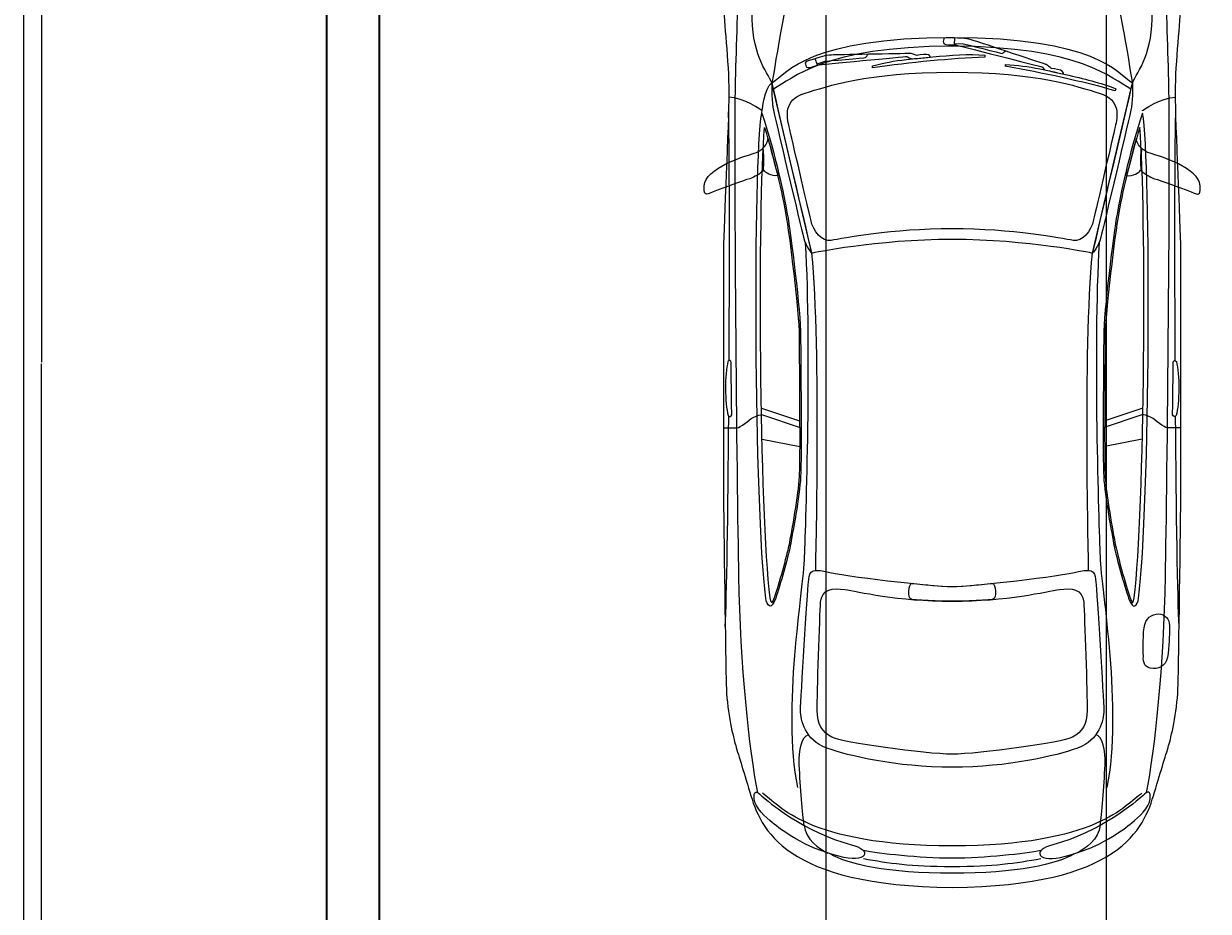
# Model space of a CAD drawing. Units: inches. Extents: x 2460 to 3031, y 933 to 2010.
# Tile 2 of 7: x 2460 to 2663, y 1104 to 1256. Entities that reach past the tile are written whole.
import ezdxf

# ---------------------------------------------------------------- set-up
doc = ezdxf.new("R2010")
doc.units = ezdxf.units.IN
for name, color, linetype, lineweight in [('A-ANNO-DIMS', 2, 'Continuous', 18), ('A-ANNO-TTLB', 7, 'Continuous', 25), ('AUDI', 7, 'Continuous', 25), ('C-PROP', 7, 'Continuous', 35)]:
    doc.layers.add(name, color=color, linetype=linetype, lineweight=lineweight)
doc.styles.get("Standard").update_dxf_attribs({"font": 'arial.ttf'})
doc.dimstyles.get("Standard").update_dxf_attribs({"dimtxt": 0.18, "dimasz": 0.18, "dimexe": 0.18, "dimexo": 0.0625, "dimgap": 0.09, "dimtad": 0, "dimtih": 1, "dimtoh": 1, "dimdec": 4, "dimzin": 0, "dimdsep": 46, "dimtxsty": 'Standard', "dimcen": 0.09, "dimadec": 0, "dimazin": 0, "dimtfac": 1, "dimtdec": 4, "dimtofl": 0, "dimtmove": 0, "dimatfit": 3, "dimfxl": 1, "dimtolj": 1, "dimtzin": 0, "dimarcsym": 0})

# ---------------------------------------------------------------- blocks, each defined once
blk = doc.blocks.new('*D35')
at = {"layer": 'A-ANNO-DIMS', "color": 0, "lineweight": -2, "transparency": 16777216}
for p, q in [((2520.61, 1339.48), (2462.69, 1339.48)), ((2462.87, 1339.3), (2462.87, 1197.91)), ((2462.87, 1056.16), (2462.87, 1197.55)), ((2511.61, 1055.98), (2462.69, 1055.98))]:
    blk.add_line(p, q, dxfattribs=at)
at = {"layer": 'A-ANNO-DIMS', "color": 0, "transparency": 16777216}
for points in [[(2462.84, 1339.3), (2462.9, 1339.3), (2462.87, 1339.48)], [(2462.84, 1056.16), (2462.9, 1056.16), (2462.87, 1055.98)]]:
    blk.add_solid(points, dxfattribs=at)
at = {"layer": 'Defpoints', "color": 0, "transparency": 16777216}
for p in [(2462.87, 1339.48), (2520.67, 1339.48), (2511.67, 1055.98)]:
    blk.add_point(p, dxfattribs=at)
at = {"layer": 'A-ANNO-DIMS', "color": 0, "transparency": 16777216, "insert": (2462.87, 1197.73), "char_height": 0.18, "attachment_point": 5}
blk.add_mtext('\\A1;283.5', dxfattribs=at)
blk = doc.blocks.new('*D37')
at = {"layer": 'A-ANNO-DIMS', "color": 0, "lineweight": -2, "transparency": 16777216}
for p, q in [((2597.17, 1554.98), (2597.17, 933.16)), ((2645.17, 1554.98), (2645.17, 933.16)), ((2597.35, 933.34), (2620.95, 933.34)), ((2644.99, 933.34), (2621.39, 933.34))]:
    blk.add_line(p, q, dxfattribs=at)
at = {"layer": 'A-ANNO-DIMS', "color": 0, "transparency": 16777216}
for points in [[(2597.35, 933.37), (2597.35, 933.31), (2597.17, 933.34)], [(2644.99, 933.37), (2644.99, 933.31), (2645.17, 933.34)]]:
    blk.add_solid(points, dxfattribs=at)
at = {"layer": 'Defpoints', "color": 0, "transparency": 16777216}
for p in [(2597.17, 1555.05), (2645.17, 1555.05), (2645.17, 933.34)]:
    blk.add_point(p, dxfattribs=at)
at = {"layer": 'A-ANNO-DIMS', "color": 0, "transparency": 16777216, "insert": (2621.17, 933.34), "char_height": 0.18, "attachment_point": 5}
blk.add_mtext('\\A1;48', dxfattribs=at)
blk = doc.blocks.new('*D40')
at = {"layer": 'A-ANNO-DIMS', "color": 0, "lineweight": -2, "transparency": 16777216}
for p, q in [((2511.67, 1056.05), (2511.67, 2006.96)), ((2511.85, 2006.78), (2516.02, 2006.78)), ((2520.49, 2006.78), (2516.32, 2006.78)), ((2520.67, 1056.05), (2520.67, 2006.96))]:
    blk.add_line(p, q, dxfattribs=at)
at = {"layer": 'A-ANNO-DIMS', "color": 0, "transparency": 16777216}
for points in [[(2511.85, 2006.81), (2511.85, 2006.75), (2511.67, 2006.78)], [(2520.49, 2006.81), (2520.49, 2006.75), (2520.67, 2006.78)]]:
    blk.add_solid(points, dxfattribs=at)
at = {"layer": 'Defpoints', "color": 0, "transparency": 16777216}
for p in [(2520.67, 2006.78), (2511.67, 1055.98), (2520.67, 1055.98)]:
    blk.add_point(p, dxfattribs=at)
at = {"layer": 'A-ANNO-DIMS', "color": 0, "transparency": 16777216, "insert": (2516.17, 2006.78), "char_height": 0.18, "attachment_point": 5}
blk.add_mtext('\\A1;9', dxfattribs=at)

msp = doc.modelspace()

# ---------------------------------------------------------------- linework, layer by layer
at = {"layer": 'A-ANNO-TTLB'}
msp.add_lwpolyline([(2459.8083, 2009.7942), (3030.6598, 2009.7942), (3030.6598, 936.3732), (2459.8083, 936.3732)], close=True, dxfattribs=at)
at = {"layer": 'AUDI'}
for points, knots in [([(2618.7829, 1107.9984), (2590.0793, 1108.312), (2585.9116, 1117.9641), (2584.1504, 1124.3238), (2584.1504, 1124.3238), (2583.0016, 1128.0786), (2582.0829, 1131.0667), (2581.6233, 1132.5994), (2581.6233, 1132.5994), (2581.1637, 1134.1318), (2580.1686, 1138.8059), (2580.0917, 1142.7138), (2580.0917, 1142.7138), (2580.0148, 1146.6218), (2579.6356, 1169.9218), (2579.6356, 1176.3523), (2579.6356, 1176.3523), (2579.6356, 1182.7825), (2579.6356, 1212.908), (2579.6356, 1217.1935), (2579.6356, 1217.1935), (2579.6356, 1221.4788), (2580.5514, 1238.5719), (2580.5514, 1244.012), (2580.5514, 1244.012), (2580.5514, 1249.4525), (2579.6356, 1256.2783), (2579.6356, 1259.1067), (2579.6356, 1259.1067), (2579.6356, 1261.9354), (2580.1681, 1276.8837), (2580.3981, 1280.1787), (2580.3981, 1280.1787), (2580.6281, 1283.4737), (2581.862, 1285.3424), (2582.9257, 1287.6881), (2582.9257, 1287.6881), (2587.0611, 1296.8058), (2597.6292, 1301.7862), (2598.7781, 1302.5527), (2598.7781, 1302.5527), (2599.9268, 1303.3191), (2601.1463, 1303.7354), (2602.6072, 1303.7354), (2602.6072, 1303.7354), (2604.0679, 1303.7354), (2604.4451, 1303.0127), (2605.0579, 1303.1658), (2605.0579, 1303.1658), (2605.6706, 1303.3191), (2607.1971, 1303.7354), (2608.8874, 1303.7354), (2608.8874, 1303.7354), (2610.5778, 1303.7354), (2618.7829, 1303.7354), (2618.7829, 1303.7354), (2618.7829, 1303.7354), (2618.7829, 1303.7354), (2626.988, 1303.7354), (2628.6784, 1303.7354), (2628.6784, 1303.7354), (2630.3689, 1303.7354), (2631.8952, 1303.3191), (2632.508, 1303.1658), (2632.508, 1303.1658), (2633.1208, 1303.0127), (2633.4979, 1303.7354), (2634.9587, 1303.7354), (2634.9587, 1303.7354), (2636.4196, 1303.7354), (2637.6391, 1303.3191), (2638.7878, 1302.5527), (2638.7878, 1302.5527), (2639.9365, 1301.7863), (2650.5047, 1296.8058), (2654.6402, 1287.6881), (2654.6402, 1287.6881), (2655.7038, 1285.3424), (2656.9377, 1283.4736), (2657.1677, 1280.1787), (2657.1677, 1280.1787), (2657.3978, 1276.8839), (2657.9302, 1261.9353), (2657.9302, 1259.1067), (2657.9302, 1259.1067), (2657.9302, 1256.2784), (2657.0145, 1249.4525), (2657.0145, 1244.012), (2657.0145, 1244.012), (2657.0145, 1238.5719), (2657.9302, 1221.4787), (2657.9302, 1217.1935), (2657.9302, 1217.1935), (2657.9302, 1212.908), (2657.9302, 1182.7824), (2657.9302, 1176.3523), (2657.9302, 1176.3523), (2657.9302, 1169.9218), (2657.5509, 1146.6216), (2657.4742, 1142.7138), (2657.4742, 1142.7138), (2657.3974, 1138.8059), (2656.4022, 1134.1318), (2655.9426, 1132.5994), (2655.9426, 1132.5994), (2655.4829, 1131.0667), (2654.5642, 1128.0785), (2653.4155, 1124.3238), (2653.4155, 1124.3238), (2651.6543, 1117.9641), (2647.4866, 1108.312), (2618.7829, 1107.9984)], [0, 0, 0, 0, 0.03571429, 0.03571429, 0.03571429, 0.0357143, 0.07142857, 0.07142857, 0.07142857, 0.07142858, 0.10714286, 0.10714286, 0.10714286, 0.10714287, 0.14285714, 0.14285714, 0.14285714, 0.14285715, 0.17857143, 0.17857143, 0.17857143, 0.17857144, 0.21428571, 0.21428571, 0.21428571, 0.21428572, 0.25, 0.25, 0.25, 0.25000001, 0.28571429, 0.28571429, 0.28571429, 0.2857143, 0.32142857, 0.32142857, 0.32142857, 0.32142858, 0.35714286, 0.35714286, 0.35714286, 0.35714287, 0.39285714, 0.39285714, 0.39285714, 0.39285715, 0.42857143, 0.42857143, 0.42857143, 0.42857144, 0.46428571, 0.46428571, 0.46428571, 0.46428572, 0.5, 0.5, 0.5, 0.50000001, 0.53571429, 0.53571429, 0.53571429, 0.5357143, 0.57142857, 0.57142857, 0.57142857, 0.57142858, 0.60714286, 0.60714286, 0.60714286, 0.60714287, 0.64285714, 0.64285714, 0.64285714, 0.64285715, 0.67857143, 0.67857143, 0.67857143, 0.67857144, 0.71428571, 0.71428571, 0.71428571, 0.71428572, 0.75, 0.75, 0.75, 0.75000001, 0.78571429, 0.78571429, 0.78571429, 0.7857143, 0.82142857, 0.82142857, 0.82142857, 0.82142858, 0.85714286, 0.85714286, 0.85714286, 0.85714287, 0.89285714, 0.89285714, 0.89285714, 0.89285715, 0.92857143, 0.92857143, 0.92857143, 0.92857144, 0.96428571, 0.96428571, 0.96428571, 0.96428572, 1, 1, 1, 1]), ([(2587.9301, 1245.7186), (2587.0363, 1247.5072), (2584.263, 1251.0766), (2584.5585, 1257.8216), (2584.5585, 1257.8216), (2584.8541, 1264.5669), (2586.0517, 1283.1771), (2587.1263, 1289.0978)], [0, 0, 0, 0, 0.5, 0.5, 0.5, 0.50000001, 1, 1, 1, 1]), ([(2649.6356, 1245.7186), (2650.5296, 1247.5072), (2653.3028, 1251.0766), (2653.0074, 1257.8216), (2653.0074, 1257.8216), (2652.7118, 1264.5669), (2651.5142, 1283.1771), (2650.4396, 1289.0978)], [0, 0, 0, 0, 0.5, 0.5, 0.5, 0.50000001, 1, 1, 1, 1]), ([(2585.4965, 1124.2398), (2584.0544, 1131.455), (2582.5189, 1146.0668), (2582.2566, 1161.2842), (2582.2566, 1161.2842), (2581.9943, 1176.5015), (2581.3391, 1235.0091), (2581.7324, 1247.34), (2581.7324, 1247.34), (2582.1256, 1259.6711), (2582.3457, 1275.227), (2584.5301, 1285.8147)], [0, 0, 0, 0, 0.33333333, 0.33333333, 0.33333333, 0.33333334, 0.66666667, 0.66666667, 0.66666667, 0.66666668, 1, 1, 1, 1]), ([(2652.0694, 1124.2398), (2653.5115, 1131.455), (2655.047, 1146.0668), (2655.3092, 1161.2842), (2655.3092, 1161.2842), (2655.5716, 1176.5015), (2656.2267, 1235.0091), (2655.8335, 1247.34), (2655.8335, 1247.34), (2655.4402, 1259.6711), (2655.2202, 1275.227), (2653.0358, 1285.8147)], [0, 0, 0, 0, 0.33333333, 0.33333333, 0.33333333, 0.33333334, 0.66666667, 0.66666667, 0.66666667, 0.66666668, 1, 1, 1, 1]), ([(2618.7829, 1218.8888), (2631.7756, 1218.8888), (2642.7845, 1216.5384), (2642.7845, 1216.5384), (2642.7845, 1216.5384), (2642.7845, 1216.5384), (2649.6356, 1245.7186), (2649.6356, 1245.7186), (2649.6356, 1245.7186), (2646.895, 1247.4815), (2643.3244, 1253.4548), (2618.7829, 1253.4548), (2618.7829, 1253.4548), (2594.2415, 1253.4548), (2590.6707, 1247.4815), (2587.9303, 1245.7186), (2587.9303, 1245.7186), (2587.9303, 1245.7186), (2594.7813, 1216.5384), (2594.7813, 1216.5384), (2594.7813, 1216.5384), (2594.7813, 1216.5384), (2605.7903, 1218.8886), (2618.7829, 1218.8888)], [0, 0, 0, 0, 0.16666667, 0.16666667, 0.16666667, 0.16666668, 0.33333333, 0.33333333, 0.33333333, 0.33333334, 0.5, 0.5, 0.5, 0.50000001, 0.66666667, 0.66666667, 0.66666667, 0.66666668, 0.83333333, 0.83333333, 0.83333333, 0.83333334, 1, 1, 1, 1]), ([(2618.7829, 1218.8888), (2631.7756, 1218.8888), (2642.7845, 1216.5384), (2642.7845, 1216.5384), (2642.7845, 1216.5384), (2642.7845, 1216.5384), (2649.6356, 1245.7186), (2649.6356, 1245.7186), (2649.6356, 1245.7186), (2646.895, 1247.4815), (2643.3244, 1253.4548), (2618.7829, 1253.4548), (2618.7829, 1253.4548), (2594.2415, 1253.4548), (2590.6707, 1247.4815), (2587.9303, 1245.7186), (2587.9303, 1245.7186), (2587.9303, 1245.7186), (2594.7813, 1216.5384), (2594.7813, 1216.5384), (2594.7813, 1216.5384), (2594.7813, 1216.5384), (2605.7903, 1218.8888), (2618.7829, 1218.8888)], [0, 0, 0, 0, 0.16666667, 0.16666667, 0.16666667, 0.16666668, 0.33333333, 0.33333333, 0.33333333, 0.33333334, 0.5, 0.5, 0.5, 0.50000001, 0.66666667, 0.66666667, 0.66666667, 0.66666668, 0.83333333, 0.83333333, 0.83333333, 0.83333334, 1, 1, 1, 1]), ([(2649.3768, 1244.617), (2646.0401, 1246.3912), (2640.8837, 1251.9486), (2618.7829, 1251.9486), (2618.7829, 1251.9486), (2596.6822, 1251.9486), (2591.5257, 1246.3912), (2588.1891, 1244.6168)], [0, 0, 0, 0, 0.5, 0.5, 0.5, 0.50000001, 1, 1, 1, 1]), ([(2619.672, 1253.3532), (2620.8626, 1253.3532), (2621.7312, 1253.1598), (2622.7614, 1252.8377), (2622.7614, 1252.8377), (2623.5334, 1252.6126), (2634.9246, 1248.8131), (2634.9246, 1248.8131), (2634.9246, 1248.8131), (2634.9246, 1248.8131), (2635.6972, 1248.2013), (2635.6972, 1248.2013), (2635.6972, 1248.2013), (2635.6972, 1248.2013), (2636.7268, 1248.0082), (2637.306, 1247.8799), (2637.306, 1247.8799), (2637.8856, 1247.719), (2637.821, 1247.2034), (2637.821, 1247.2034), (2637.821, 1247.2034), (2637.821, 1247.2034), (2634.6672, 1247.9118), (2634.6672, 1247.9118), (2634.6672, 1247.9118), (2634.6672, 1247.9118), (2634.1526, 1248.4273), (2634.1526, 1248.4273), (2634.1526, 1248.4273), (2634.1526, 1248.4273), (2619.3499, 1252.194), (2619.3499, 1252.194), (2619.3499, 1252.194), (2619.3499, 1252.194), (2618.8671, 1252.1939), (2618.127, 1252.1939), (2618.127, 1252.1939), (2617.3866, 1252.2259), (2617.2584, 1252.4837), (2617.2584, 1252.7731), (2617.2584, 1252.7731), (2617.2584, 1253.0953), (2617.2907, 1253.3855), (2617.7411, 1253.3855), (2617.7411, 1253.3855), (2618.1915, 1253.4175), (2618.9317, 1253.3855), (2619.672, 1253.3532)], [0, 0, 0, 0, 0.08333333, 0.08333333, 0.08333333, 0.08333334, 0.16666667, 0.16666667, 0.16666667, 0.16666668, 0.25, 0.25, 0.25, 0.25000001, 0.33333333, 0.33333333, 0.33333333, 0.33333334, 0.41666667, 0.41666667, 0.41666667, 0.41666668, 0.5, 0.5, 0.5, 0.50000001, 0.58333333, 0.58333333, 0.58333333, 0.58333334, 0.66666667, 0.66666667, 0.66666667, 0.66666668, 0.75, 0.75, 0.75, 0.75000001, 0.83333333, 0.83333333, 0.83333333, 0.83333334, 0.91666667, 0.91666667, 0.91666667, 0.91666668, 1, 1, 1, 1]), ([(2619.1893, 1252.4193), (2619.1893, 1252.4193), (2620.6693, 1252.387), (2620.6693, 1252.387), (2620.6693, 1252.387), (2620.6693, 1252.387), (2627.3624, 1250.7126), (2627.3624, 1250.7126), (2627.3624, 1250.7126), (2627.3624, 1250.7126), (2627.9098, 1251.1312), (2627.9098, 1251.1312)], [0, 0, 0, 0, 0.33333333, 0.33333333, 0.33333333, 0.33333334, 0.66666667, 0.66666667, 0.66666667, 0.66666668, 1, 1, 1, 1]), ([(2595.7944, 1249.972), (2596.8886, 1250.3588), (2597.7895, 1250.455), (2598.8837, 1250.4873), (2598.8837, 1250.4873), (2599.6881, 1250.4875), (2611.7877, 1250.7126), (2611.7877, 1250.7126), (2611.7877, 1250.7126), (2611.7877, 1250.7126), (2612.7208, 1250.3906), (2612.7208, 1250.3906), (2612.7208, 1250.3906), (2612.7208, 1250.3906), (2613.7828, 1250.5197), (2614.362, 1250.552), (2614.362, 1250.552), (2614.9416, 1250.6162), (2615.0376, 1250.1011), (2615.0376, 1250.1011), (2615.0376, 1250.1011), (2615.0376, 1250.1011), (2611.8524, 1249.779), (2611.8524, 1249.779), (2611.8524, 1249.779), (2611.8524, 1249.779), (2610.9834, 1250.1976), (2610.9834, 1250.1976), (2610.9834, 1250.1976), (2610.9834, 1250.1976), (2595.859, 1248.7808), (2595.859, 1248.7808), (2595.859, 1248.7808), (2595.859, 1248.7808), (2595.4086, 1248.6202), (2594.7006, 1248.3949), (2594.7006, 1248.3949), (2594.0245, 1248.1694), (2593.7994, 1248.3626), (2593.7028, 1248.6525), (2593.7028, 1248.6525), (2593.6059, 1248.9738), (2593.5418, 1249.2326), (2593.9604, 1249.3927), (2593.9604, 1249.3927), (2594.3785, 1249.5216), (2595.0864, 1249.7467), (2595.7944, 1249.972)], [0, 0, 0, 0, 0.08333333, 0.08333333, 0.08333333, 0.08333334, 0.16666667, 0.16666667, 0.16666667, 0.16666668, 0.25, 0.25, 0.25, 0.25000001, 0.33333333, 0.33333333, 0.33333333, 0.33333334, 0.41666667, 0.41666667, 0.41666667, 0.41666668, 0.5, 0.5, 0.5, 0.50000001, 0.58333333, 0.58333333, 0.58333333, 0.58333334, 0.66666667, 0.66666667, 0.66666667, 0.66666668, 0.75, 0.75, 0.75, 0.75000001, 0.83333333, 0.83333333, 0.83333333, 0.83333334, 0.91666667, 0.91666667, 0.91666667, 0.91666668, 1, 1, 1, 1]), ([(2595.7944, 1249.972), (2596.8886, 1250.3588), (2597.7895, 1250.455), (2598.8837, 1250.4873), (2598.8837, 1250.4873), (2599.6881, 1250.4873), (2611.7877, 1250.7126), (2611.7877, 1250.7126), (2611.7877, 1250.7126), (2611.7877, 1250.7126), (2612.7208, 1250.3906), (2612.7208, 1250.3906), (2612.7208, 1250.3906), (2612.7208, 1250.3906), (2613.7828, 1250.5197), (2614.362, 1250.552), (2614.362, 1250.552), (2614.9416, 1250.6162), (2615.0376, 1250.1011), (2615.0376, 1250.1011), (2615.0376, 1250.1011), (2615.0376, 1250.1011), (2611.8524, 1249.779), (2611.8524, 1249.779), (2611.8524, 1249.779), (2611.8524, 1249.779), (2610.9834, 1250.1976), (2610.9834, 1250.1976), (2610.9834, 1250.1976), (2610.9834, 1250.1976), (2595.859, 1248.7808), (2595.859, 1248.7808), (2595.859, 1248.7808), (2595.859, 1248.7808), (2595.4086, 1248.6202), (2594.7006, 1248.3949), (2594.7006, 1248.3949), (2594.0245, 1248.1694), (2593.7994, 1248.3626), (2593.7028, 1248.6525), (2593.7028, 1248.6525), (2593.6059, 1248.9738), (2593.5418, 1249.2326), (2593.9604, 1249.3927), (2593.9604, 1249.3927), (2594.3785, 1249.5216), (2595.0864, 1249.7467), (2595.7944, 1249.972)], [0, 0, 0, 0, 0.08333333, 0.08333333, 0.08333333, 0.08333334, 0.16666667, 0.16666667, 0.16666667, 0.16666668, 0.25, 0.25, 0.25, 0.25000001, 0.33333333, 0.33333333, 0.33333333, 0.33333334, 0.41666667, 0.41666667, 0.41666667, 0.41666668, 0.5, 0.5, 0.5, 0.50000001, 0.58333333, 0.58333333, 0.58333333, 0.58333334, 0.66666667, 0.66666667, 0.66666667, 0.66666668, 0.75, 0.75, 0.75, 0.75000001, 0.83333333, 0.83333333, 0.83333333, 0.83333334, 0.91666667, 0.91666667, 0.91666667, 0.91666668, 1, 1, 1, 1]), ([(2595.666, 1248.942), (2595.666, 1248.942), (2597.0492, 1249.3929), (2597.0492, 1249.3929), (2597.0492, 1249.3929), (2597.0492, 1249.3929), (2603.9681, 1250.0043), (2603.9681, 1250.0043), (2603.9681, 1250.0043), (2603.9681, 1250.0043), (2604.3543, 1250.5521), (2604.3543, 1250.5521)], [0, 0, 0, 0, 0.33333333, 0.33333333, 0.33333333, 0.33333334, 0.66666667, 0.66666667, 0.66666667, 0.66666668, 1, 1, 1, 1]), ([(2624.3701, 1250.4552), (2621.6025, 1250.6481), (2618.5774, 1250.4227), (2615.4558, 1250.1334), (2615.4558, 1250.1334), (2613.9439, 1249.972), (2612.4311, 1249.8436), (2610.9511, 1249.6821), (2610.9511, 1249.6821), (2608.8595, 1249.4893), (2607.0897, 1249.0706), (2605.1587, 1248.6202), (2605.1587, 1248.6202), (2605.1587, 1248.6202), (2605.1587, 1248.2654), (2605.1587, 1248.2654), (2605.1587, 1248.2654), (2611.7231, 1249.1999), (2618.5455, 1249.8436), (2624.4024, 1250.1011), (2624.4024, 1250.1011), (2624.4024, 1250.1011), (2624.3701, 1250.4552), (2624.3701, 1250.4552)], [0, 0, 0, 0, 0.16666667, 0.16666667, 0.16666667, 0.16666668, 0.33333333, 0.33333333, 0.33333333, 0.33333334, 0.5, 0.5, 0.5, 0.50000001, 0.66666667, 0.66666667, 0.66666667, 0.66666668, 0.83333333, 0.83333333, 0.83333333, 0.83333334, 1, 1, 1, 1]), ([(2618.7829, 1220.7249), (2629.0961, 1220.7249), (2637.5374, 1219.0336), (2639.4913, 1218.7381), (2639.4913, 1218.7381), (2641.0857, 1218.4968), (2642.5602, 1220.2217), (2643.0071, 1222.29), (2643.0071, 1222.29), (2643.454, 1224.3581), (2646.3033, 1236.4318), (2646.6944, 1238.1647), (2646.6944, 1238.1647), (2647.0855, 1239.8976), (2647.7558, 1242.7484), (2643.9568, 1243.9221), (2643.9568, 1243.9221), (2640.1579, 1245.0962), (2633.4425, 1247.4993), (2618.7829, 1247.4993), (2618.7829, 1247.4993), (2604.1234, 1247.4993), (2597.408, 1245.0961), (2593.6091, 1243.9221), (2593.6091, 1243.9221), (2589.81, 1242.7485), (2590.4804, 1239.8975), (2590.8715, 1238.1647), (2590.8715, 1238.1647), (2591.2625, 1236.432), (2594.1118, 1224.358), (2594.5587, 1222.29), (2594.5587, 1222.29), (2595.0057, 1220.2218), (2596.4801, 1218.4968), (2598.0744, 1218.7381), (2598.0744, 1218.7381), (2600.0285, 1219.0337), (2608.4697, 1220.7249), (2618.7829, 1220.7249)], [0, 0, 0, 0, 0.1, 0.1, 0.1, 0.10000001, 0.2, 0.2, 0.2, 0.20000001, 0.3, 0.3, 0.3, 0.30000001, 0.4, 0.4, 0.4, 0.40000001, 0.5, 0.5, 0.5, 0.50000001, 0.6, 0.6, 0.6, 0.60000001, 0.7, 0.7, 0.7, 0.70000001, 0.8, 0.8, 0.8, 0.80000001, 0.9, 0.9, 0.9, 0.90000001, 1, 1, 1, 1]), ([(2646.7991, 1244.6921), (2644.2248, 1245.6898), (2641.2962, 1246.4304), (2638.2069, 1247.1065), (2638.2069, 1247.1065), (2636.7268, 1247.4286), (2635.2468, 1247.7826), (2633.7986, 1248.0724), (2633.7986, 1248.0724), (2631.7713, 1248.5243), (2629.9368, 1248.6843), (2627.9422, 1248.8454), (2627.9422, 1248.8454), (2627.9422, 1248.8454), (2627.8452, 1248.5243), (2627.8452, 1248.5243), (2627.8452, 1248.5243), (2634.3778, 1247.3965), (2641.0391, 1245.9154), (2646.7026, 1244.338), (2646.7026, 1244.338), (2646.7026, 1244.338), (2646.7991, 1244.6921), (2646.7991, 1244.6921)], [0, 0, 0, 0, 0.16666667, 0.16666667, 0.16666667, 0.16666668, 0.33333333, 0.33333333, 0.33333333, 0.33333334, 0.5, 0.5, 0.5, 0.50000001, 0.66666667, 0.66666667, 0.66666667, 0.66666668, 0.83333333, 0.83333333, 0.83333333, 0.83333334, 1, 1, 1, 1]), ([(2587.9301, 1245.7186), (2587.9301, 1245.7186), (2594.7813, 1216.5384), (2594.7813, 1216.5384), (2594.7813, 1216.5384), (2594.7813, 1216.5384), (2593.7103, 1217.5998), (2593.3188, 1219.2645), (2593.3188, 1219.2645), (2592.9272, 1220.9292), (2588.3828, 1239.9489), (2588.089, 1241.5154), (2588.089, 1241.5154), (2587.7953, 1243.082), (2587.9303, 1245.7186), (2587.9301, 1245.7186)], [0, 0, 0, 0, 0.25, 0.25, 0.25, 0.25000001, 0.5, 0.5, 0.5, 0.50000001, 0.75, 0.75, 0.75, 0.75000001, 1, 1, 1, 1]), ([(2587.9301, 1245.7186), (2587.9301, 1245.7186), (2594.7813, 1216.5384), (2594.7813, 1216.5384), (2594.7813, 1216.5384), (2594.7813, 1216.5384), (2593.7103, 1217.5998), (2593.3188, 1219.2645), (2593.3188, 1219.2645), (2592.9272, 1220.9292), (2588.3828, 1239.9489), (2588.089, 1241.5154), (2588.089, 1241.5154), (2587.7953, 1243.082), (2587.9301, 1245.7186), (2587.9301, 1245.7186)], [0, 0, 0, 0, 0.25, 0.25, 0.25, 0.25000001, 0.5, 0.5, 0.5, 0.50000001, 0.75, 0.75, 0.75, 0.75000001, 1, 1, 1, 1]), ([(2649.6356, 1245.7186), (2649.6356, 1245.7186), (2642.7845, 1216.5384), (2642.7845, 1216.5384), (2642.7845, 1216.5384), (2642.7845, 1216.5384), (2643.8556, 1217.5998), (2644.2471, 1219.2645), (2644.2471, 1219.2645), (2644.6385, 1220.9292), (2649.1831, 1239.9489), (2649.4768, 1241.5154), (2649.4768, 1241.5154), (2649.7706, 1243.082), (2649.6356, 1245.7186), (2649.6356, 1245.7186)], [0, 0, 0, 0, 0.25, 0.25, 0.25, 0.25000001, 0.5, 0.5, 0.5, 0.50000001, 0.75, 0.75, 0.75, 0.75000001, 1, 1, 1, 1]), ([(2586.8744, 1157.4941), (2587.0272, 1156.2939), (2587.7696, 1155.2062), (2588.5648, 1157.4941), (2588.5648, 1157.4941), (2589.3601, 1159.7819), (2590.6525, 1164.4571), (2591.05, 1166.4463), (2591.05, 1166.4463), (2591.4476, 1168.4352), (2592.6409, 1174.9998), (2592.8395, 1178.2823), (2592.8395, 1178.2823), (2593.0382, 1181.5647), (2592.8395, 1198.3743), (2592.8395, 1202.3528), (2592.8395, 1202.3528), (2592.8395, 1206.3316), (2591.1496, 1219.9584), (2590.5529, 1223.2406), (2590.5529, 1223.2406), (2589.9563, 1226.5229), (2588.6639, 1233.0877), (2586.1752, 1240.4823), (2586.1752, 1240.4823), (2584.6877, 1232.2922), (2584.8859, 1173.1101), (2586.8744, 1157.4941)], [0, 0, 0, 0, 0.14285714, 0.14285714, 0.14285714, 0.14285715, 0.28571429, 0.28571429, 0.28571429, 0.2857143, 0.42857143, 0.42857143, 0.42857143, 0.42857144, 0.57142857, 0.57142857, 0.57142857, 0.57142858, 0.71428571, 0.71428571, 0.71428571, 0.71428572, 0.85714286, 0.85714286, 0.85714286, 0.85714287, 1, 1, 1, 1]), ([(2650.6915, 1157.4941), (2650.5387, 1156.2939), (2649.7963, 1155.2062), (2649.001, 1157.4941), (2649.001, 1157.4941), (2648.2058, 1159.7819), (2646.9135, 1164.4571), (2646.5159, 1166.4463), (2646.5159, 1166.4463), (2646.1183, 1168.4352), (2644.9249, 1174.9998), (2644.7263, 1178.2823), (2644.7263, 1178.2823), (2644.5277, 1181.5647), (2644.7263, 1198.3743), (2644.7263, 1202.3528), (2644.7263, 1202.3528), (2644.7263, 1206.3316), (2646.4163, 1219.9584), (2647.013, 1223.2406), (2647.013, 1223.2406), (2647.6096, 1226.5229), (2648.902, 1233.0877), (2651.3907, 1240.4823), (2651.3907, 1240.4823), (2652.8782, 1232.2922), (2652.68, 1173.1101), (2650.6915, 1157.4941)], [0, 0, 0, 0, 0.14285714, 0.14285714, 0.14285714, 0.14285715, 0.28571429, 0.28571429, 0.28571429, 0.2857143, 0.42857143, 0.42857143, 0.42857143, 0.42857144, 0.57142857, 0.57142857, 0.57142857, 0.57142858, 0.71428571, 0.71428571, 0.71428571, 0.71428572, 0.85714286, 0.85714286, 0.85714286, 0.85714287, 1, 1, 1, 1]), ([(2587.6304, 1157.5581), (2587.6304, 1157.5581), (2587.6304, 1157.5581), (2587.6304, 1157.5581), (2587.6304, 1157.5581), (2587.6862, 1157.1186), (2587.8058, 1156.8635), (2587.8926, 1156.7406), (2587.8926, 1156.7406), (2587.9835, 1156.8489), (2588.1402, 1157.0879), (2588.3392, 1157.6607), (2588.3392, 1157.6607), (2589.1143, 1159.8904), (2590.4054, 1164.5405), (2590.806, 1166.5455), (2590.806, 1166.5455), (2591.2862, 1168.9474), (2592.4013, 1175.2447), (2592.5868, 1178.3128), (2592.5868, 1178.3128), (2592.7321, 1180.7132), (2592.6623, 1190.5221), (2592.6164, 1197.013), (2592.6164, 1197.013), (2592.6164, 1197.013), (2592.5859, 1202.3529), (2592.5859, 1202.3529), (2592.5859, 1202.3529), (2592.5859, 1206.3203), (2590.8776, 1220.0125), (2590.3076, 1223.1499), (2590.3076, 1223.1499), (2589.3539, 1228.3963), (2588.117, 1233.392), (2586.654, 1238.0769), (2586.654, 1238.0769), (2585.4851, 1224.5051), (2585.7875, 1172.0275), (2587.6304, 1157.5581)], [0, 0, 0, 0, 0.1, 0.1, 0.1, 0.10000001, 0.2, 0.2, 0.2, 0.20000001, 0.3, 0.3, 0.3, 0.30000001, 0.4, 0.4, 0.4, 0.40000001, 0.5, 0.5, 0.5, 0.50000001, 0.6, 0.6, 0.6, 0.60000001, 0.7, 0.7, 0.7, 0.70000001, 0.8, 0.8, 0.8, 0.80000001, 0.9, 0.9, 0.9, 0.90000001, 1, 1, 1, 1]), ([(2649.9355, 1157.5581), (2649.9355, 1157.5581), (2649.9355, 1157.5581), (2649.9355, 1157.5581), (2649.9355, 1157.5581), (2649.8796, 1157.1186), (2649.76, 1156.8635), (2649.6733, 1156.7406), (2649.6733, 1156.7406), (2649.5824, 1156.8489), (2649.4257, 1157.0879), (2649.2267, 1157.6607), (2649.2267, 1157.6607), (2648.4516, 1159.8904), (2647.1605, 1164.5405), (2646.7599, 1166.5455), (2646.7599, 1166.5455), (2646.2797, 1168.9474), (2645.1646, 1175.2447), (2644.9791, 1178.3128), (2644.9791, 1178.3128), (2644.8337, 1180.7132), (2644.9036, 1190.5221), (2644.9493, 1197.013), (2644.9493, 1197.013), (2644.9493, 1197.013), (2644.98, 1202.3529), (2644.98, 1202.3529), (2644.98, 1202.3529), (2644.98, 1206.3203), (2646.6883, 1220.0125), (2647.2583, 1223.1499), (2647.2583, 1223.1499), (2648.2119, 1228.3963), (2649.4489, 1233.392), (2650.9119, 1238.0769), (2650.9119, 1238.0769), (2652.0808, 1224.5051), (2651.7782, 1172.0275), (2649.9355, 1157.5581)], [0, 0, 0, 0, 0.1, 0.1, 0.1, 0.10000001, 0.2, 0.2, 0.2, 0.20000001, 0.3, 0.3, 0.3, 0.30000001, 0.4, 0.4, 0.4, 0.40000001, 0.5, 0.5, 0.5, 0.50000001, 0.6, 0.6, 0.6, 0.60000001, 0.7, 0.7, 0.7, 0.70000001, 0.8, 0.8, 0.8, 0.80000001, 0.9, 0.9, 0.9, 0.90000001, 1, 1, 1, 1]), ([(2586.341, 1234.4618), (2586.499, 1233.6439), (2586.5135, 1231.8626), (2586.4178, 1230.6365), (2586.4178, 1230.6365), (2586.4532, 1230.6755), (2586.4924, 1230.7151), (2586.5165, 1230.75), (2586.5165, 1230.75), (2586.7364, 1230.283), (2587.8687, 1229.6668), (2588.9096, 1229.8374), (2588.9096, 1229.8374), (2588.773, 1230.4084), (2587.2523, 1236.0998), (2587.2523, 1236.0998), (2587.2523, 1236.0998), (2587.1904, 1235.6289), (2586.894, 1234.9895), (2586.341, 1234.4618)], [0, 0, 0, 0, 0.2, 0.2, 0.2, 0.20000001, 0.4, 0.4, 0.4, 0.40000001, 0.6, 0.6, 0.6, 0.60000001, 0.8, 0.8, 0.8, 0.80000001, 1, 1, 1, 1]), ([(2651.2248, 1234.4618), (2651.0669, 1233.6439), (2651.0524, 1231.8626), (2651.1481, 1230.6365), (2651.1481, 1230.6365), (2651.1127, 1230.6755), (2651.0735, 1230.7151), (2651.0494, 1230.75), (2651.0494, 1230.75), (2650.8294, 1230.283), (2649.6972, 1229.6668), (2648.6563, 1229.8374), (2648.6563, 1229.8374), (2648.7929, 1230.4084), (2650.3136, 1236.0998), (2650.3136, 1236.0998), (2650.3136, 1236.0998), (2650.3755, 1235.6289), (2650.6718, 1234.9895), (2651.2248, 1234.4618)], [0, 0, 0, 0, 0.2, 0.2, 0.2, 0.20000001, 0.4, 0.4, 0.4, 0.40000001, 0.6, 0.6, 0.6, 0.60000001, 0.8, 0.8, 0.8, 0.80000001, 1, 1, 1, 1]), ([(2586.341, 1234.4618), (2585.97, 1234.1074), (2585.4864, 1233.8022), (2584.8684, 1233.6364), (2584.8684, 1233.6364), (2583.3298, 1233.2235), (2576.4075, 1231.0529), (2576.3251, 1228.0841), (2576.3251, 1228.0841), (2576.3251, 1226.8198), (2576.3522, 1226.3801), (2577.3411, 1226.8196), (2577.3411, 1226.8196), (2578.3302, 1227.2596), (2583.3029, 1229.0456), (2584.1269, 1229.2932), (2584.1269, 1229.2932), (2584.8855, 1229.5215), (2586.0071, 1230.1882), (2586.4178, 1230.6365), (2586.4178, 1230.6365), (2586.5135, 1231.8626), (2586.499, 1233.6439), (2586.341, 1234.4618)], [0, 0, 0, 0, 0.16666667, 0.16666667, 0.16666667, 0.16666668, 0.33333333, 0.33333333, 0.33333333, 0.33333334, 0.5, 0.5, 0.5, 0.50000001, 0.66666667, 0.66666667, 0.66666667, 0.66666668, 0.83333333, 0.83333333, 0.83333333, 0.83333334, 1, 1, 1, 1]), ([(2651.2248, 1234.4618), (2651.5958, 1234.1074), (2652.0794, 1233.8022), (2652.6975, 1233.6364), (2652.6975, 1233.6364), (2654.2359, 1233.2235), (2661.1583, 1231.0529), (2661.2408, 1228.0841), (2661.2408, 1228.0841), (2661.2408, 1226.8198), (2661.2137, 1226.3801), (2660.2247, 1226.8196), (2660.2247, 1226.8196), (2659.2357, 1227.2596), (2654.263, 1229.0456), (2653.439, 1229.2932), (2653.439, 1229.2932), (2652.6804, 1229.5215), (2651.5587, 1230.1882), (2651.1481, 1230.6365), (2651.1481, 1230.6365), (2651.0524, 1231.8626), (2651.0669, 1233.6439), (2651.2248, 1234.4618)], [0, 0, 0, 0, 0.16666667, 0.16666667, 0.16666667, 0.16666668, 0.33333333, 0.33333333, 0.33333333, 0.33333334, 0.5, 0.5, 0.5, 0.50000001, 0.66666667, 0.66666667, 0.66666667, 0.66666668, 0.83333333, 0.83333333, 0.83333333, 0.83333334, 1, 1, 1, 1]), ([(2593.6309, 1218.3227), (2594.6596, 1199.7579), (2593.6915, 1170.563), (2593.4681, 1164.638), (2593.4681, 1164.638), (2593.2446, 1158.713), (2589.618, 1138.5888), (2592.2756, 1125.1233)], [0, 0, 0, 0, 0.5, 0.5, 0.5, 0.50000001, 1, 1, 1, 1]), ([(2643.935, 1218.3227), (2642.9063, 1199.7579), (2643.8743, 1170.563), (2644.0978, 1164.638), (2644.0978, 1164.638), (2644.3213, 1158.713), (2647.9479, 1138.5888), (2645.2902, 1125.1233)], [0, 0, 0, 0, 0.5, 0.5, 0.5, 0.50000001, 1, 1, 1, 1]), ([(2581.0384, 1188.9052), (2581.0384, 1188.5544), (2580.5587, 1188.4227), (2580.4523, 1188.7737), (2580.4523, 1188.7737), (2580.1319, 1189.7827), (2579.973, 1191.5807), (2579.973, 1193.3791), (2579.973, 1193.3791), (2579.973, 1195.1775), (2580.0791, 1196.9318), (2580.3986, 1197.9844), (2580.3986, 1197.9844), (2580.505, 1198.2915), (2580.9311, 1198.2036), (2580.9311, 1197.8527), (2580.9311, 1197.8527), (2580.9311, 1197.8527), (2581.0384, 1188.9052), (2581.0384, 1188.9052)], [0, 0, 0, 0, 0.2, 0.2, 0.2, 0.20000001, 0.4, 0.4, 0.4, 0.40000001, 0.6, 0.6, 0.6, 0.60000001, 0.8, 0.8, 0.8, 0.80000001, 1, 1, 1, 1]), ([(2656.5274, 1188.9052), (2656.5274, 1188.5544), (2657.007, 1188.4227), (2657.1136, 1188.7737), (2657.1136, 1188.7737), (2657.434, 1189.7827), (2657.5929, 1191.5807), (2657.5929, 1193.3791), (2657.5929, 1193.3791), (2657.5929, 1195.1775), (2657.4868, 1196.9318), (2657.1673, 1197.9844), (2657.1673, 1197.9844), (2657.0608, 1198.2915), (2656.6348, 1198.2036), (2656.6348, 1197.8527), (2656.6348, 1197.8527), (2656.6348, 1197.8527), (2656.5274, 1188.9052), (2656.5274, 1188.9052)], [0, 0, 0, 0, 0.2, 0.2, 0.2, 0.20000001, 0.4, 0.4, 0.4, 0.40000001, 0.6, 0.6, 0.6, 0.60000001, 0.8, 0.8, 0.8, 0.80000001, 1, 1, 1, 1]), ([(2579.6356, 1186.6527), (2579.6356, 1186.6527), (2581.3605, 1186.6525), (2581.9271, 1186.6525), (2581.9271, 1186.6525), (2582.4935, 1186.6525), (2583.9951, 1188.0264), (2584.6877, 1188.4279), (2584.6877, 1188.4279), (2585.3803, 1188.8295), (2586.1411, 1188.9246), (2586.1411, 1188.9246)], [0, 0, 0, 0, 0.33333333, 0.33333333, 0.33333333, 0.33333334, 0.66666667, 0.66666667, 0.66666667, 0.66666668, 1, 1, 1, 1]), ([(2657.9302, 1186.6527), (2657.9302, 1186.6527), (2656.2053, 1186.6525), (2655.6388, 1186.6525), (2655.6388, 1186.6525), (2655.0722, 1186.6525), (2653.5709, 1188.0264), (2652.8782, 1188.4279), (2652.8782, 1188.4279), (2652.1855, 1188.8295), (2651.4248, 1188.9246), (2651.4248, 1188.9246)], [0, 0, 0, 0, 0.33333333, 0.33333333, 0.33333333, 0.33333334, 0.66666667, 0.66666667, 0.66666667, 0.66666668, 1, 1, 1, 1]), ([(2618.7829, 1128.5883), (2628.4331, 1128.5883), (2636.5453, 1130.5258), (2640.2696, 1131.8674), (2640.2696, 1131.8674), (2643.9939, 1133.2089), (2644.739, 1136.6373), (2644.739, 1138.3513), (2644.739, 1138.3513), (2644.739, 1140.0656), (2643.547, 1158.9215), (2643.3981, 1160.2631), (2643.3981, 1160.2631), (2643.2494, 1161.6046), (2643.3235, 1162.7972), (2640.4185, 1162.0517), (2640.4185, 1162.0517), (2637.5133, 1161.3063), (2622.3921, 1159.5178), (2618.7829, 1159.5178), (2618.7829, 1159.5178), (2615.1738, 1159.5179), (2600.0526, 1161.3063), (2597.1474, 1162.0517), (2597.1474, 1162.0517), (2594.2423, 1162.7972), (2594.3165, 1161.6046), (2594.1676, 1160.2631), (2594.1676, 1160.2631), (2594.0189, 1158.9215), (2592.8269, 1140.0655), (2592.8269, 1138.3513), (2592.8269, 1138.3513), (2592.8269, 1136.6373), (2593.5719, 1133.2089), (2597.2963, 1131.8674), (2597.2963, 1131.8674), (2601.0205, 1130.5258), (2609.1327, 1128.5883), (2618.7829, 1128.5883)], [0, 0, 0, 0, 0.1, 0.1, 0.1, 0.10000001, 0.2, 0.2, 0.2, 0.20000001, 0.3, 0.3, 0.3, 0.30000001, 0.4, 0.4, 0.4, 0.40000001, 0.5, 0.5, 0.5, 0.50000001, 0.6, 0.6, 0.6, 0.60000001, 0.7, 0.7, 0.7, 0.70000001, 0.8, 0.8, 0.8, 0.80000001, 0.9, 0.9, 0.9, 0.90000001, 1, 1, 1, 1]), ([(2618.7829, 1128.5883), (2628.4331, 1128.5883), (2636.5453, 1130.5258), (2640.2696, 1131.8674), (2640.2696, 1131.8674), (2643.9939, 1133.2089), (2644.739, 1136.6373), (2644.739, 1138.3513), (2644.739, 1138.3513), (2644.739, 1140.0656), (2643.547, 1158.9215), (2643.3981, 1160.2631), (2643.3981, 1160.2631), (2643.2494, 1161.6046), (2643.3235, 1162.7972), (2640.4185, 1162.0517), (2640.4185, 1162.0517), (2637.5133, 1161.3063), (2622.3921, 1159.5178), (2618.7829, 1159.5178), (2618.7829, 1159.5178), (2615.1738, 1159.5178), (2600.0526, 1161.3063), (2597.1474, 1162.0517), (2597.1474, 1162.0517), (2594.2423, 1162.7972), (2594.3165, 1161.6046), (2594.1676, 1160.2631), (2594.1676, 1160.2631), (2594.0189, 1158.9215), (2592.8269, 1140.0655), (2592.8269, 1138.3513), (2592.8269, 1138.3513), (2592.8269, 1136.6373), (2593.5719, 1133.2089), (2597.2963, 1131.8674), (2597.2963, 1131.8674), (2601.0205, 1130.5258), (2609.1327, 1128.5883), (2618.7829, 1128.5883)], [0, 0, 0, 0, 0.1, 0.1, 0.1, 0.10000001, 0.2, 0.2, 0.2, 0.20000001, 0.3, 0.3, 0.3, 0.30000001, 0.4, 0.4, 0.4, 0.40000001, 0.5, 0.5, 0.5, 0.50000001, 0.6, 0.6, 0.6, 0.60000001, 0.7, 0.7, 0.7, 0.70000001, 0.8, 0.8, 0.8, 0.80000001, 0.9, 0.9, 0.9, 0.90000001, 1, 1, 1, 1]), ([(2618.7829, 1130.8193), (2623.3605, 1130.8193), (2637.7368, 1132.8363), (2639.3757, 1133.7307), (2639.3757, 1133.7307), (2641.0147, 1134.625), (2641.9085, 1135.8919), (2641.9085, 1138.3513), (2641.9085, 1138.3513), (2641.9085, 1140.8108), (2641.4611, 1154.5989), (2641.3123, 1156.8347), (2641.3123, 1156.8347), (2641.1634, 1159.0707), (2639.1523, 1159.2943), (2637.1411, 1158.9961), (2637.1411, 1158.9961), (2635.1297, 1158.698), (2628.0534, 1156.984), (2618.7829, 1156.984), (2618.7829, 1156.984), (2609.5124, 1156.984), (2602.436, 1158.698), (2600.4248, 1158.9961), (2600.4248, 1158.9961), (2598.4136, 1159.2943), (2596.4024, 1159.0707), (2596.2535, 1156.8347), (2596.2535, 1156.8347), (2596.1046, 1154.599), (2595.6573, 1140.8108), (2595.6573, 1138.3513), (2595.6573, 1138.3513), (2595.6573, 1135.8919), (2596.5512, 1134.625), (2598.1901, 1133.7307), (2598.1901, 1133.7307), (2599.829, 1132.8365), (2614.2053, 1130.8193), (2618.7829, 1130.8193)], [0, 0, 0, 0, 0.1, 0.1, 0.1, 0.10000001, 0.2, 0.2, 0.2, 0.20000001, 0.3, 0.3, 0.3, 0.30000001, 0.4, 0.4, 0.4, 0.40000001, 0.5, 0.5, 0.5, 0.50000001, 0.6, 0.6, 0.6, 0.60000001, 0.7, 0.7, 0.7, 0.70000001, 0.8, 0.8, 0.8, 0.80000001, 0.9, 0.9, 0.9, 0.90000001, 1, 1, 1, 1]), ([(2618.7829, 1156.984), (2618.7829, 1156.984), (2624.2487, 1157.08), (2625.6743, 1157.2902), (2625.6743, 1157.2902), (2626.5659, 1157.4218), (2626.1466, 1160.0883), (2625.7297, 1160.048), (2625.7297, 1160.048), (2623.1104, 1159.7937), (2620.9081, 1159.5178), (2618.7829, 1159.5178), (2618.7829, 1159.5178), (2616.6578, 1159.5178), (2614.4554, 1159.7937), (2611.8363, 1160.048), (2611.8363, 1160.048), (2611.4193, 1160.0884), (2611, 1157.4217), (2611.8916, 1157.2902), (2611.8916, 1157.2902), (2613.317, 1157.08), (2618.7829, 1156.984), (2618.7829, 1156.984)], [0, 0, 0, 0, 0.16666667, 0.16666667, 0.16666667, 0.16666668, 0.33333333, 0.33333333, 0.33333333, 0.33333334, 0.5, 0.5, 0.5, 0.50000001, 0.66666667, 0.66666667, 0.66666667, 0.66666668, 0.83333333, 0.83333333, 0.83333333, 0.83333334, 1, 1, 1, 1]), ([(2651.526, 1147.4845), (2651.4225, 1146.5105), (2651.7713, 1145.5008), (2653.1845, 1145.4738), (2653.1845, 1145.4738), (2654.5979, 1145.4467), (2655.5686, 1146.1994), (2655.7759, 1148.0662), (2655.7759, 1148.0662), (2655.9831, 1149.9327), (2655.9831, 1151.7992), (2655.9831, 1152.8365), (2655.9831, 1152.8365), (2655.9831, 1153.8736), (2655.2573, 1154.8066), (2654.1173, 1154.8066), (2654.1173, 1154.8066), (2652.9772, 1154.8066), (2651.8373, 1154.0811), (2651.6299, 1152.4218), (2651.6299, 1152.4218), (2651.4225, 1150.7624), (2651.526, 1147.4845), (2651.526, 1147.4845)], [0, 0, 0, 0, 0.16666667, 0.16666667, 0.16666667, 0.16666668, 0.33333333, 0.33333333, 0.33333333, 0.33333334, 0.5, 0.5, 0.5, 0.50000001, 0.66666667, 0.66666667, 0.66666667, 0.66666668, 0.83333333, 0.83333333, 0.83333333, 0.83333334, 1, 1, 1, 1]), ([(2593.424, 1118.6474), (2593.204, 1120.486), (2592.7688, 1125.1904), (2592.6034, 1128.9981), (2592.6034, 1128.9981), (2592.4916, 1131.5693), (2593.0434, 1133.8613), (2594.1642, 1134.1685)], [0, 0, 0, 0, 0.5, 0.5, 0.5, 0.50000001, 1, 1, 1, 1]), ([(2644.1419, 1118.6474), (2644.3619, 1120.486), (2644.797, 1125.1904), (2644.9625, 1128.9981), (2644.9625, 1128.9981), (2645.0742, 1131.5693), (2644.5225, 1133.8613), (2643.4017, 1134.1685)], [0, 0, 0, 0, 0.5, 0.5, 0.5, 0.50000001, 1, 1, 1, 1]), ([(2601.5517, 1115.3318), (2593.5937, 1117.3901), (2587.1486, 1122.7541), (2586.1547, 1123.7191), (2586.1547, 1123.7191), (2585.28, 1124.5686), (2584.7427, 1124.6617), (2584.8793, 1123.1656), (2584.8793, 1123.1656), (2585.0142, 1121.6894), (2586.8753, 1120.0265), (2588.0175, 1119.0791), (2588.0175, 1119.0791), (2589.4765, 1117.8688), (2593.482, 1114.8473), (2599.3996, 1113.3405), (2599.3996, 1113.3405), (2601.6592, 1112.6945), (2603.2732, 1112.9098), (2603.7036, 1113.5556), (2603.7036, 1113.5556), (2604.1339, 1114.2016), (2603.1322, 1114.9211), (2601.5517, 1115.3318)], [0, 0, 0, 0, 0.16666667, 0.16666667, 0.16666667, 0.16666668, 0.33333333, 0.33333333, 0.33333333, 0.33333334, 0.5, 0.5, 0.5, 0.50000001, 0.66666667, 0.66666667, 0.66666667, 0.66666668, 0.83333333, 0.83333333, 0.83333333, 0.83333334, 1, 1, 1, 1]), ([(2651.2741, 1124.133), (2648.4262, 1122.1786), (2643.5544, 1115.1355), (2618.7829, 1115.1355), (2618.7829, 1115.1355), (2594.0114, 1115.1355), (2589.1396, 1122.1786), (2586.2918, 1124.133)], [0, 0, 0, 0, 0.5, 0.5, 0.5, 0.50000001, 1, 1, 1, 1]), ([(2636.014, 1115.3318), (2643.9722, 1117.3901), (2650.4174, 1122.7541), (2651.4112, 1123.7191), (2651.4112, 1123.7191), (2652.2859, 1124.5686), (2652.8232, 1124.6617), (2652.6865, 1123.1656), (2652.6865, 1123.1656), (2652.5517, 1121.6894), (2650.6906, 1120.0265), (2649.5485, 1119.0791), (2649.5485, 1119.0791), (2648.0892, 1117.8688), (2644.0839, 1114.8473), (2638.1663, 1113.3405), (2638.1663, 1113.3405), (2635.9067, 1112.6945), (2634.2927, 1112.9098), (2633.8623, 1113.5556), (2633.8623, 1113.5556), (2633.4319, 1114.2016), (2634.4337, 1114.9211), (2636.014, 1115.3318)], [0, 0, 0, 0, 0.16666667, 0.16666667, 0.16666667, 0.16666668, 0.33333333, 0.33333333, 0.33333333, 0.33333334, 0.5, 0.5, 0.5, 0.50000001, 0.66666667, 0.66666667, 0.66666667, 0.66666668, 0.83333333, 0.83333333, 0.83333333, 0.83333334, 1, 1, 1, 1]), ([(2639.6834, 1113.7718), (2636.9176, 1112.0058), (2629.6994, 1110.4407), (2618.7829, 1110.4407), (2618.7829, 1110.4407), (2607.8665, 1110.4407), (2600.6483, 1112.0058), (2597.8825, 1113.7718)], [0, 0, 0, 0, 0.5, 0.5, 0.5, 0.50000001, 1, 1, 1, 1]), ([(2633.9819, 1114.3414), (2631.1073, 1113.7941), (2624.5595, 1113.0116), (2618.7829, 1113.0116), (2618.7829, 1113.0116), (2613.0063, 1113.0116), (2606.4585, 1113.7941), (2603.584, 1114.3414)], [0, 0, 0, 0, 0.5, 0.5, 0.5, 0.50000001, 1, 1, 1, 1]), ([(2633.9819, 1112.8998), (2629.543, 1112.1175), (2626.012, 1111.5585), (2618.7829, 1111.5585), (2618.7829, 1111.5585), (2611.5537, 1111.5585), (2608.0227, 1112.1175), (2603.584, 1112.8998)], [0, 0, 0, 0, 0.5, 0.5, 0.5, 0.50000001, 1, 1, 1, 1])]:
    msp.add_open_spline(points, degree=3, knots=knots, dxfattribs=at)
for points in [[(2598.5576, 1298.6599), (2596.0301, 1290.615), (2588.3637, 1249.4001), (2587.9167, 1245.3755)], [(2639.0083, 1298.6599), (2641.5358, 1290.615), (2649.2022, 1249.4001), (2649.6492, 1245.3755)], [(2619.1893, 1252.194), (2619.1893, 1252.194), (2619.2211, 1253.3855), (2619.2211, 1253.3855)], [(2595.7303, 1248.7167), (2595.7303, 1248.7167), (2595.3435, 1249.8436), (2595.3435, 1249.8436)], [(2586.1227, 1240.0092), (2586.2716, 1241.351), (2586.5885, 1244.6886), (2587.9303, 1245.7186)], [(2586.2297, 1240.9463), (2586.2297, 1240.9463), (2583.0144, 1243.2132), (2580.546, 1243.2132)], [(2651.3362, 1240.9463), (2651.3362, 1240.9463), (2654.5516, 1243.2132), (2657.0198, 1243.2132)], [(2580.5858, 1198.1614), (2580.684, 1215.9431), (2580.6727, 1233.625), (2580.4925, 1240.7441)], [(2656.9801, 1198.1614), (2656.8819, 1215.9431), (2656.8933, 1233.625), (2657.0734, 1240.7441)], [(2595.4099, 1162.2685), (2595.4099, 1162.2685), (2596.3636, 1200.2967), (2594.7813, 1216.5384)], [(2642.156, 1162.2685), (2642.156, 1162.2685), (2641.2023, 1200.2967), (2642.7845, 1216.5384)], [(2579.9246, 1152.6938), (2580.179, 1157.2341), (2580.395, 1172.1507), (2580.523, 1188.6489)], [(2586.1219, 1190.0083), (2586.1219, 1190.0083), (2592.6693, 1187.8586), (2592.6693, 1187.8586)], [(2586.1411, 1188.9246), (2586.1411, 1188.9246), (2592.9259, 1186.6527), (2592.9259, 1186.6527)], [(2651.4248, 1188.9246), (2651.4248, 1188.9246), (2644.6399, 1186.6527), (2644.6399, 1186.6527)], [(2651.444, 1190.0083), (2651.444, 1190.0083), (2644.8966, 1187.8586), (2644.8966, 1187.8586)], [(2657.6413, 1152.6938), (2657.3869, 1157.2341), (2657.1707, 1172.1507), (2657.0429, 1188.6489)], [(2586.2275, 1184.7419), (2586.2275, 1184.7419), (2592.6719, 1183.454), (2592.6719, 1183.454)], [(2651.3382, 1184.7419), (2651.3382, 1184.7419), (2644.894, 1183.454), (2644.894, 1183.454)], [(2593.424, 1118.6474), (2593.6749, 1116.2927), (2595.9843, 1114.6133), (2597.4866, 1113.8989)], [(2644.1419, 1118.6474), (2643.8909, 1116.2927), (2641.5816, 1114.6133), (2640.0793, 1113.8989)]]:
    msp.add_open_spline(points, degree=3, dxfattribs=at)
at = {"layer": 'C-PROP'}
for p, q in [((2511.6684, 1957.9828), (2511.6684, 1055.9828)), ((2511.6684, 1957.9828), (2511.6684, 1055.9828)), ((2520.6684, 1339.4828), (2520.6684, 1055.9828))]:
    msp.add_line(p, q, dxfattribs=at)

# ---------------------------------------------------------------- dimensions: what is measured, and where the dimension line sits
at = {"layer": 'A-ANNO-DIMS'}
for base, p1, p2, picture, middle in [((2520.6684, 2006.7823), (2511.6684, 1055.9828), (2520.6684, 1055.9828), '*D40', (2516.1684, 2006.7823)), ((2645.1684, 933.3411), (2597.1684, 1555.0454), (2645.1684, 1555.0454), '*D37', (2621.1684, 933.3411))]:
    dim = msp.add_linear_dim(base=base, p1=p1, p2=p2, dimstyle='Standard', override={"dimdec": 0, "dimlfac": 1, "dimrnd": 0, "dimzin": 0, "dimdsep": 46, "dimlunit": 2}, dxfattribs=at)
    dim.commit()
    dim.dimension.update_dxf_attribs({"geometry": picture, "text_midpoint": middle})
dim = msp.add_linear_dim(base=(2462.8689, 1339.4828), p1=(2511.6684, 1055.9828), p2=(2520.6684, 1339.4828), angle=90, dimstyle='Standard', override={"dimdec": 1, "dimlfac": 1, "dimrnd": 0, "dimzin": 0, "dimdsep": 46, "dimlunit": 2}, dxfattribs=at)
dim.commit()
dim.dimension.update_dxf_attribs({"geometry": '*D35', "text_midpoint": (2462.8689, 1197.7328)})

doc.saveas('drawing.dxf')
